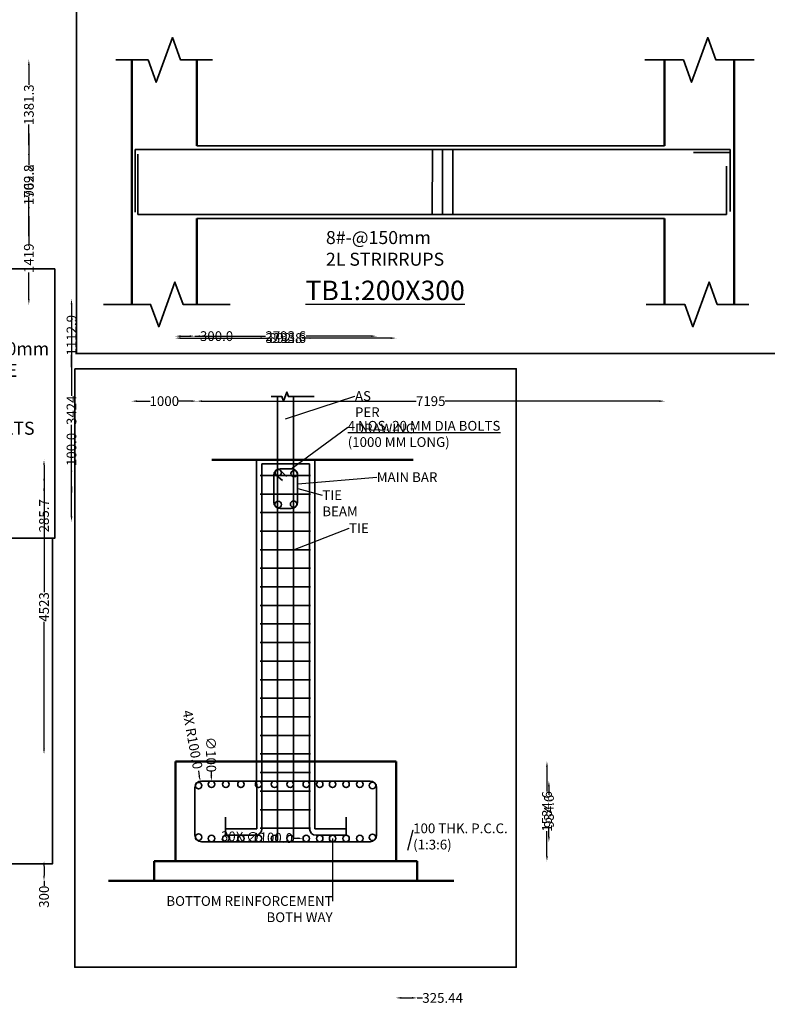
# Model space of a CAD drawing. Units: millimetres. Extents: x -19888 to 14444, y 67066 to 90098.
# Tile 3 of 7: x -9513 to 1986, y 67066 to 82214. Entities that reach past the tile are written whole.
import ezdxf
from ezdxf import colors
from ezdxf.entities.mleader import LeaderData, LeaderLine
from ezdxf.math import Vec2, Vec3

# ---------------------------------------------------------------- set-up
doc = ezdxf.new("R2010")
doc.units = ezdxf.units.MM
doc.header["$LTSCALE"] = 50
doc.header["$MEASUREMENT"] = 0
for name, color, linetype, lineweight in [('S-ANNO-DIMS', 2, 'Continuous', 18), ('S-ANNO-TEXT', 7, 'Continuous', 25), ('S-ANNO-TTLB', 7, 'Continuous', 35), ('S-BEAM', 3, 'Continuous', 35), ('S-COLS', 4, 'Continuous', 50), ('S-FNDN', 1, 'Continuous', 50), ('S-REIN', 6, 'Continuous', 35)]:
    doc.layers.add(name, color=color, linetype=linetype, lineweight=lineweight)
doc.styles.get("Standard").update_dxf_attribs({"font": 'arial.ttf'})
doc.dimstyles.get("Standard").update_dxf_attribs({"dimtxt": 150, "dimasz": 80, "dimexe": 0.18, "dimexo": 0.0625, "dimgap": 0.09, "dimtad": 0, "dimdec": 0, "dimzin": 0, "dimdsep": 46, "dimtxsty": 'Standard', "dimcen": 0.09, "dimadec": 0, "dimazin": 0, "dimtfac": 1, "dimtdec": 0, "dimtofl": 0, "dimtmove": 0, "dimatfit": 3, "dimfxl": 1, "dimfxlon": 1, "dimtolj": 1, "dimtzin": 0, "dimarcsym": 0})

# ---------------------------------------------------------------- blocks, each defined once
blk = doc.blocks.new('*D41')
at = {"layer": 'Defpoints', "color": 0, "ltscale": 50, "transparency": 16777216}
for p in [(-11742, 77917), (-8716, 77917), (-11519, 74493)]:
    blk.add_point(p, dxfattribs=at)
at = {"layer": 'S-ANNO-DIMS', "color": 0, "lineweight": -2, "ltscale": 50, "transparency": 16777216}
for p, q in [((-8717, 77917), (-8716, 77917)), ((-8716, 77837), (-8716, 76429)), ((-8716, 74573), (-8716, 75981)), ((-8717, 74493), (-8716, 74493))]:
    blk.add_line(p, q, dxfattribs=at)
at = {"layer": 'S-ANNO-DIMS', "color": 0, "ltscale": 50, "transparency": 16777216}
for points in [[(-8729, 77837), (-8703, 77837), (-8716, 77917)], [(-8729, 74573), (-8703, 74573), (-8716, 74493)]]:
    blk.add_solid(points, dxfattribs=at)
at = {"layer": 'S-ANNO-DIMS', "color": 0, "ltscale": 50, "transparency": 16777216, "insert": (-8716, 76205), "char_height": 150, "attachment_point": 5, "rotation": 90}
blk.add_mtext('\\A1;3424', dxfattribs=at)
blk = doc.blocks.new('*D42')
at = {"layer": 'Defpoints', "color": 0, "ltscale": 50, "transparency": 16777216}
for p in [(-11742, 77917), (-11219, 76804), (-8716, 76804)]:
    blk.add_point(p, dxfattribs=at)
at = {"layer": 'S-ANNO-DIMS', "color": 0, "lineweight": -2, "ltscale": 50, "transparency": 16777216}
for p, q in [((-8717, 77917), (-8716, 77917)), ((-8716, 77837), (-8716, 77665)), ((-8716, 76884), (-8716, 77056)), ((-8717, 76804), (-8716, 76804))]:
    blk.add_line(p, q, dxfattribs=at)
at = {"layer": 'S-ANNO-DIMS', "color": 0, "ltscale": 50, "transparency": 16777216}
for points in [[(-8729, 77837), (-8703, 77837), (-8716, 77917)], [(-8729, 76884), (-8703, 76884), (-8716, 76804)]]:
    blk.add_solid(points, dxfattribs=at)
at = {"layer": 'S-ANNO-DIMS', "color": 0, "ltscale": 50, "transparency": 16777216, "insert": (-8716, 77360), "char_height": 150, "attachment_point": 5, "rotation": 90}
blk.add_mtext('\\A1;1112.9', dxfattribs=at)
blk = doc.blocks.new('*D51')
at = {"layer": 'Defpoints', "color": 0, "ltscale": 50, "transparency": 16777216}
for p in [(1476, 82673), (-7789, 81597), (1476, 81597)]:
    blk.add_point(p, dxfattribs=at)
at = {"layer": 'S-ANNO-DIMS', "color": 0, "lineweight": -2, "ltscale": 50, "transparency": 16777216}
for p, q in [((-7789, 82672), (-7789, 82673)), ((-7709, 82673), (-3381, 82673)), ((1396, 82673), (-2931, 82673)), ((1476, 82672), (1476, 82673))]:
    blk.add_line(p, q, dxfattribs=at)
at = {"layer": 'S-ANNO-DIMS', "color": 0, "ltscale": 50, "transparency": 16777216}
for points in [[(-7709, 82686), (-7709, 82659), (-7789, 82673)], [(1396, 82686), (1396, 82659), (1476, 82673)]]:
    blk.add_solid(points, dxfattribs=at)
at = {"layer": 'S-ANNO-DIMS', "color": 0, "ltscale": 50, "transparency": 16777216, "insert": (-3156, 82673), "char_height": 150, "attachment_point": 5}
blk.add_mtext('\\A1;9265', dxfattribs=at)
blk = doc.blocks.new('*D52')
at = {"layer": 'Defpoints', "color": 0, "ltscale": 50, "transparency": 16777216}
for p in [(-7789, 77834), (-6789, 77834), (-6789, 76346)]:
    blk.add_point(p, dxfattribs=at)
at = {"layer": 'S-ANNO-DIMS', "color": 0, "lineweight": -2, "ltscale": 50, "transparency": 16777216}
for p, q in [((-7789, 76347), (-7789, 76346)), ((-7709, 76346), (-7505, 76346)), ((-6869, 76346), (-7072, 76346)), ((-6789, 76347), (-6789, 76346))]:
    blk.add_line(p, q, dxfattribs=at)
at = {"layer": 'S-ANNO-DIMS', "color": 0, "ltscale": 50, "transparency": 16777216}
for points in [[(-7709, 76359), (-7709, 76333), (-7789, 76346)], [(-6869, 76359), (-6869, 76333), (-6789, 76346)]]:
    blk.add_solid(points, dxfattribs=at)
at = {"layer": 'S-ANNO-DIMS', "color": 0, "ltscale": 50, "transparency": 16777216, "insert": (-7289, 76346), "char_height": 150, "attachment_point": 5}
blk.add_mtext('\\A1;1000', dxfattribs=at)
blk = doc.blocks.new('*D53')
at = {"layer": 'Defpoints', "color": 0, "ltscale": 50, "transparency": 16777216}
for p in [(-6789, 77834), (407, 77834), (407, 76346)]:
    blk.add_point(p, dxfattribs=at)
at = {"layer": 'S-ANNO-DIMS', "color": 0, "lineweight": -2, "ltscale": 50, "transparency": 16777216}
for p, q in [((-6789, 76347), (-6789, 76346)), ((-6709, 76346), (-3415, 76346)), ((327, 76346), (-2967, 76346)), ((407, 76347), (407, 76346))]:
    blk.add_line(p, q, dxfattribs=at)
at = {"layer": 'S-ANNO-DIMS', "color": 0, "ltscale": 50, "transparency": 16777216}
for points in [[(-6709, 76359), (-6709, 76333), (-6789, 76346)], [(327, 76359), (327, 76333), (407, 76346)]]:
    blk.add_solid(points, dxfattribs=at)
at = {"layer": 'S-ANNO-DIMS', "color": 0, "ltscale": 50, "transparency": 16777216, "insert": (-3191, 76346), "char_height": 150, "attachment_point": 5}
blk.add_mtext('\\A1;7195', dxfattribs=at)
blk = doc.blocks.new('*D54')
at = {"layer": 'Defpoints', "color": 0, "ltscale": 50, "transparency": 16777216}
for p in [(-7789, 81597), (-9372, 80215), (-7739, 80215)]:
    blk.add_point(p, dxfattribs=at)
at = {"layer": 'S-ANNO-DIMS', "color": 0, "lineweight": -2, "ltscale": 50, "transparency": 16777216}
for p, q in [((-9371, 81597), (-9372, 81597)), ((-9372, 81517), (-9372, 81210)), ((-9372, 80295), (-9372, 80602)), ((-9371, 80215), (-9372, 80215))]:
    blk.add_line(p, q, dxfattribs=at)
at = {"layer": 'S-ANNO-DIMS', "color": 0, "ltscale": 50, "transparency": 16777216}
for points in [[(-9385, 81517), (-9359, 81517), (-9372, 81597)], [(-9385, 80295), (-9359, 80295), (-9372, 80215)]]:
    blk.add_solid(points, dxfattribs=at)
at = {"layer": 'S-ANNO-DIMS', "color": 0, "ltscale": 50, "transparency": 16777216, "insert": (-9372, 80906), "char_height": 150, "attachment_point": 5, "rotation": 90}
blk.add_mtext('\\A1;1381.3', dxfattribs=at)
blk = doc.blocks.new('*D55')
at = {"layer": 'Defpoints', "color": 0, "ltscale": 50, "transparency": 16777216}
for p in [(-7739, 80215), (-9372, 79253), (-7739, 79253)]:
    blk.add_point(p, dxfattribs=at)
at = {"layer": 'S-ANNO-DIMS', "color": 0, "lineweight": -2, "ltscale": 50, "transparency": 16777216}
for p, q in [((-9371, 80215), (-9372, 80215)), ((-9372, 80135), (-9372, 79987)), ((-9372, 79333), (-9372, 79482)), ((-9371, 79253), (-9372, 79253))]:
    blk.add_line(p, q, dxfattribs=at)
at = {"layer": 'S-ANNO-DIMS', "color": 0, "ltscale": 50, "transparency": 16777216}
for points in [[(-9385, 80135), (-9359, 80135), (-9372, 80215)], [(-9385, 79333), (-9359, 79333), (-9372, 79253)]]:
    blk.add_solid(points, dxfattribs=at)
at = {"layer": 'S-ANNO-DIMS', "color": 0, "ltscale": 50, "transparency": 16777216, "insert": (-9372, 79734), "char_height": 150, "attachment_point": 5, "rotation": 90}
blk.add_mtext('\\A1;962.2', dxfattribs=at)
blk = doc.blocks.new('*D56')
at = {"layer": 'Defpoints', "color": 0, "ltscale": 50, "transparency": 16777216}
for p in [(-7739, 79253), (-9372, 77834), (-7789, 77834)]:
    blk.add_point(p, dxfattribs=at)
at = {"layer": 'S-ANNO-DIMS', "color": 0, "lineweight": -2, "ltscale": 50, "transparency": 16777216}
for p, q in [((-9371, 79253), (-9372, 79253)), ((-9372, 79173), (-9372, 78761)), ((-9372, 77914), (-9372, 78326)), ((-9371, 77834), (-9372, 77834))]:
    blk.add_line(p, q, dxfattribs=at)
at = {"layer": 'S-ANNO-DIMS', "color": 0, "ltscale": 50, "transparency": 16777216}
for points in [[(-9385, 79173), (-9359, 79173), (-9372, 79253)], [(-9385, 77914), (-9359, 77914), (-9372, 77834)]]:
    blk.add_solid(points, dxfattribs=at)
at = {"layer": 'S-ANNO-DIMS', "color": 0, "ltscale": 50, "transparency": 16777216, "insert": (-9372, 78544), "char_height": 150, "attachment_point": 5, "rotation": 90}
blk.add_mtext('\\A1;1419', dxfattribs=at)
blk = doc.blocks.new('*D57')
at = {"layer": 'Defpoints', "color": 0, "ltscale": 50, "transparency": 16777216}
for p in [(-3161, 82673), (-6789, 80274), (-3161, 80215)]:
    blk.add_point(p, dxfattribs=at)
at = {"layer": 'S-ANNO-DIMS', "color": 0, "lineweight": -2, "ltscale": 50, "transparency": 16777216}
for p, q in [((-6789, 82672), (-6789, 82673)), ((-6709, 82673), (-5286, 82673)), ((-3241, 82673), (-4664, 82673)), ((-3161, 82672), (-3161, 82673))]:
    blk.add_line(p, q, dxfattribs=at)
at = {"layer": 'S-ANNO-DIMS', "color": 0, "ltscale": 50, "transparency": 16777216}
for points in [[(-6709, 82686), (-6709, 82659), (-6789, 82673)], [(-3241, 82686), (-3241, 82659), (-3161, 82673)]]:
    blk.add_solid(points, dxfattribs=at)
at = {"layer": 'S-ANNO-DIMS', "color": 0, "ltscale": 50, "transparency": 16777216, "insert": (-4975, 82673), "char_height": 150, "attachment_point": 5}
blk.add_mtext('\\A1;3627.4', dxfattribs=at)
blk = doc.blocks.new('*D59')
at = {"layer": 'Defpoints', "color": 0, "ltscale": 50, "transparency": 16777216}
for p in [(2744, 80527), (-9372, 78817), (2744, 78817)]:
    blk.add_point(p, dxfattribs=at)
at = {"layer": 'S-ANNO-DIMS', "color": 0, "lineweight": -2, "ltscale": 50, "transparency": 16777216}
for p, q in [((-9371, 80527), (-9372, 80527)), ((-9372, 80447), (-9372, 79976)), ((-9372, 78897), (-9372, 79367)), ((-9371, 78817), (-9372, 78817))]:
    blk.add_line(p, q, dxfattribs=at)
at = {"layer": 'S-ANNO-DIMS', "color": 0, "ltscale": 50, "transparency": 16777216}
for points in [[(-9385, 80447), (-9359, 80447), (-9372, 80527)], [(-9385, 78897), (-9359, 78897), (-9372, 78817)]]:
    blk.add_solid(points, dxfattribs=at)
at = {"layer": 'S-ANNO-DIMS', "color": 0, "ltscale": 50, "transparency": 16777216, "insert": (-9372, 79672), "char_height": 150, "attachment_point": 5, "rotation": 90}
blk.add_mtext('\\A1;1709.8', dxfattribs=at)
blk = doc.blocks.new('*D61')
at = {"layer": 'Defpoints', "color": 0, "ltscale": 50, "transparency": 16777216}
for p in [(-3725, 77316), (-7118, 70801), (-3725, 70801)]:
    blk.add_point(p, dxfattribs=at)
at = {"layer": 'S-ANNO-DIMS', "color": 0, "lineweight": -2, "ltscale": 50, "transparency": 16777216}
for p, q in [((-7118, 77315), (-7118, 77316)), ((-7038, 77316), (-5733, 77316)), ((-3805, 77316), (-5110, 77316)), ((-3725, 77315), (-3725, 77316))]:
    blk.add_line(p, q, dxfattribs=at)
at = {"layer": 'S-ANNO-DIMS', "color": 0, "ltscale": 50, "transparency": 16777216}
for points in [[(-7038, 77329), (-7038, 77302), (-7118, 77316)], [(-3805, 77329), (-3805, 77302), (-3725, 77316)]]:
    blk.add_solid(points, dxfattribs=at)
at = {"layer": 'S-ANNO-DIMS', "color": 0, "ltscale": 50, "transparency": 16777216, "insert": (-5421, 77316), "char_height": 150, "attachment_point": 5}
blk.add_mtext('\\A1;3393.6', dxfattribs=at)
blk = doc.blocks.new('*D62')
at = {"layer": 'Defpoints', "color": 0, "ltscale": 50, "transparency": 16777216}
for p in [(-3725, 69267), (-3399, 69267), (-3399, 67164)]:
    blk.add_point(p, dxfattribs=at)
at = {"layer": 'S-ANNO-DIMS', "color": 0, "lineweight": -2, "ltscale": 50, "transparency": 16777216}
for p, q in [((-3725, 67165), (-3725, 67164)), ((-3645, 67164), (-3479, 67164)), ((-3399, 67165), (-3399, 67164)), ((-3399, 67164), (-3319, 67164))]:
    blk.add_line(p, q, dxfattribs=at)
at = {"layer": 'S-ANNO-DIMS', "color": 0, "ltscale": 50, "transparency": 16777216}
for points in [[(-3645, 67178), (-3645, 67151), (-3725, 67164)], [(-3479, 67178), (-3479, 67151), (-3399, 67164)]]:
    blk.add_solid(points, dxfattribs=at)
at = {"layer": 'S-ANNO-DIMS', "color": 0, "ltscale": 50, "transparency": 16777216, "insert": (-3008, 67164), "char_height": 150, "attachment_point": 5}
blk.add_mtext('\\A1;325.44', dxfattribs=at)
blk = doc.blocks.new('*D63')
at = {"layer": 'Defpoints', "color": 0, "ltscale": 50, "transparency": 16777216}
for p in [(-4975, 77316), (-5868, 69767), (-4975, 69767)]:
    blk.add_point(p, dxfattribs=at)
at = {"layer": 'S-ANNO-DIMS', "color": 0, "lineweight": -2, "ltscale": 50, "transparency": 16777216}
for p, q in [((-5868, 77315), (-5868, 77316)), ((-5788, 77316), (-5675, 77316)), ((-5055, 77316), (-5168, 77316)), ((-4975, 77315), (-4975, 77316))]:
    blk.add_line(p, q, dxfattribs=at)
at = {"layer": 'S-ANNO-DIMS', "color": 0, "ltscale": 50, "transparency": 16777216}
for points in [[(-5788, 77329), (-5788, 77302), (-5868, 77316)], [(-5055, 77329), (-5055, 77302), (-4975, 77316)]]:
    blk.add_solid(points, dxfattribs=at)
at = {"layer": 'S-ANNO-DIMS', "color": 0, "ltscale": 50, "transparency": 16777216, "insert": (-5421, 77316), "char_height": 150, "attachment_point": 5}
blk.add_mtext('\\A1;892.8', dxfattribs=at)
blk = doc.blocks.new('*D64')
at = {"layer": 'Defpoints', "color": 0, "ltscale": 50, "transparency": 16777216}
for p in [(-3725, 70801), (-3725, 69267), (-1403, 69267)]:
    blk.add_point(p, dxfattribs=at)
at = {"layer": 'S-ANNO-DIMS', "color": 0, "lineweight": -2, "ltscale": 50, "transparency": 16777216}
for p, q in [((-1404, 70801), (-1403, 70801)), ((-1403, 70721), (-1403, 70338)), ((-1403, 69347), (-1403, 69730)), ((-1404, 69267), (-1403, 69267))]:
    blk.add_line(p, q, dxfattribs=at)
at = {"layer": 'S-ANNO-DIMS', "color": 0, "ltscale": 50, "transparency": 16777216}
for points in [[(-1417, 70721), (-1390, 70721), (-1403, 70801)], [(-1417, 69347), (-1390, 69347), (-1403, 69267)]]:
    blk.add_solid(points, dxfattribs=at)
at = {"layer": 'S-ANNO-DIMS', "color": 0, "ltscale": 50, "transparency": 16777216, "insert": (-1403, 70034), "char_height": 150, "attachment_point": 5, "rotation": 90}
blk.add_mtext('\\A1;1534.6', dxfattribs=at)
blk = doc.blocks.new('*D65')
at = {"layer": 'Defpoints', "color": 0, "ltscale": 50, "transparency": 16777216}
for p in [(-7444, 69267), (-9139, 68967), (-7444, 68967)]:
    blk.add_point(p, dxfattribs=at)
at = {"layer": 'S-ANNO-DIMS', "color": 0, "lineweight": -2, "ltscale": 50, "transparency": 16777216}
for p, q in [((-9138, 69267), (-9139, 69267)), ((-9139, 69187), (-9139, 69047)), ((-9138, 68967), (-9139, 68967)), ((-9139, 68967), (-9139, 68887))]:
    blk.add_line(p, q, dxfattribs=at)
at = {"layer": 'S-ANNO-DIMS', "color": 0, "ltscale": 50, "transparency": 16777216}
for points in [[(-9152, 69187), (-9126, 69187), (-9139, 69267)], [(-9152, 69047), (-9126, 69047), (-9139, 68967)]]:
    blk.add_solid(points, dxfattribs=at)
at = {"layer": 'S-ANNO-DIMS', "color": 0, "ltscale": 50, "transparency": 16777216, "insert": (-9139, 68721), "char_height": 150, "attachment_point": 5, "rotation": 90}
blk.add_mtext('\\A1;300', dxfattribs=at)
blk = doc.blocks.new('*D66')
at = {"layer": 'Defpoints', "color": 0, "ltscale": 50, "transparency": 16777216}
for p in [(-5868, 75441), (-9139, 70917), (-5814, 70917)]:
    blk.add_point(p, dxfattribs=at)
at = {"layer": 'S-ANNO-DIMS', "color": 0, "lineweight": -2, "ltscale": 50, "transparency": 16777216}
for p, q in [((-9138, 75441), (-9139, 75441)), ((-9139, 75361), (-9139, 73406)), ((-9139, 70997), (-9139, 72952)), ((-9138, 70917), (-9139, 70917))]:
    blk.add_line(p, q, dxfattribs=at)
at = {"layer": 'S-ANNO-DIMS', "color": 0, "ltscale": 50, "transparency": 16777216}
for points in [[(-9152, 75361), (-9126, 75361), (-9139, 75441)], [(-9152, 70997), (-9126, 70997), (-9139, 70917)]]:
    blk.add_solid(points, dxfattribs=at)
at = {"layer": 'S-ANNO-DIMS', "color": 0, "ltscale": 50, "transparency": 16777216, "insert": (-9139, 73179), "char_height": 150, "attachment_point": 5, "rotation": 90}
blk.add_mtext('\\A1;4523', dxfattribs=at)
blk = doc.blocks.new('*D67')
at = {"layer": 'Defpoints', "color": 0, "ltscale": 50, "transparency": 16777216}
for p in [(-5814, 75202), (-9139, 74917), (-5814, 74917)]:
    blk.add_point(p, dxfattribs=at)
at = {"layer": 'S-ANNO-DIMS', "color": 0, "lineweight": -2, "ltscale": 50, "transparency": 16777216}
for p, q in [((-9138, 75202), (-9139, 75202)), ((-9139, 75122), (-9139, 74997)), ((-9138, 74917), (-9139, 74917)), ((-9139, 74917), (-9139, 74837))]:
    blk.add_line(p, q, dxfattribs=at)
at = {"layer": 'S-ANNO-DIMS', "color": 0, "ltscale": 50, "transparency": 16777216}
for points in [[(-9152, 75122), (-9126, 75122), (-9139, 75202)], [(-9152, 74997), (-9126, 74997), (-9139, 74917)]]:
    blk.add_solid(points, dxfattribs=at)
at = {"layer": 'S-ANNO-DIMS', "color": 0, "ltscale": 50, "transparency": 16777216, "insert": (-9139, 74582), "char_height": 150, "attachment_point": 5, "rotation": 90}
blk.add_mtext('\\A1;285.7', dxfattribs=at)
blk = doc.blocks.new('*D71')
at = {"layer": 'Defpoints', "color": 0, "ltscale": 50, "transparency": 16777216}
for p in [(-6564, 70501), (-6563, 70401)]:
    blk.add_point(p, dxfattribs=at)
at = {"layer": 'S-ANNO-DIMS', "color": 0, "lineweight": -2, "ltscale": 50, "transparency": 16777216}
for p, q in [((-6567, 70661), (-6566, 70581)), ((-6564, 70451), (-6563, 70451)), ((-6564, 70451), (-6564, 70451))]:
    blk.add_line(p, q, dxfattribs=at)
at = {"layer": 'S-ANNO-DIMS', "color": 0, "ltscale": 50, "transparency": 16777216}
blk.add_solid([(-6552, 70581), (-6579, 70581), (-6564, 70501)], dxfattribs=at)
at = {"layer": 'S-ANNO-DIMS', "color": 0, "ltscale": 50, "transparency": 16777216, "insert": (-6570, 70908), "char_height": 150, "attachment_point": 5, "rotation": 270.8674}
blk.add_mtext('\\A1;∅100', dxfattribs=at)
blk = doc.blocks.new('*D94')
at = {"layer": 'Defpoints', "color": 0, "ltscale": 50, "transparency": 16777216}
for p in [(-11369, 75198), (-8716, 75198), (-11369, 75098)]:
    blk.add_point(p, dxfattribs=at)
at = {"layer": 'S-ANNO-DIMS', "color": 0, "lineweight": -2, "ltscale": 50, "transparency": 16777216}
for p, q in [((-8716, 75278), (-8716, 75358)), ((-8717, 75198), (-8716, 75198)), ((-8717, 75098), (-8716, 75098)), ((-8716, 75018), (-8716, 74938))]:
    blk.add_line(p, q, dxfattribs=at)
at = {"layer": 'S-ANNO-DIMS', "color": 0, "ltscale": 50, "transparency": 16777216}
for points in [[(-8729, 75278), (-8703, 75278), (-8716, 75198)], [(-8729, 75018), (-8703, 75018), (-8716, 75098)]]:
    blk.add_solid(points, dxfattribs=at)
at = {"layer": 'S-ANNO-DIMS', "color": 0, "ltscale": 50, "transparency": 16777216, "insert": (-8716, 75603), "char_height": 150, "attachment_point": 5, "rotation": 90}
blk.add_mtext('\\A1;100.0', dxfattribs=at)
blk = doc.blocks.new('*D97')
at = {"layer": 'Defpoints', "color": 0, "ltscale": 50, "transparency": 16777216}
for p in [(-4025, 77346), (-6818, 70401), (-4025, 70401)]:
    blk.add_point(p, dxfattribs=at)
at = {"layer": 'S-ANNO-DIMS', "color": 0, "lineweight": -2, "ltscale": 50, "transparency": 16777216}
for p, q in [((-6818, 77345), (-6818, 77346)), ((-6738, 77346), (-5734, 77346)), ((-4105, 77346), (-5109, 77346)), ((-4025, 77345), (-4025, 77346))]:
    blk.add_line(p, q, dxfattribs=at)
at = {"layer": 'S-ANNO-DIMS', "color": 0, "ltscale": 50, "transparency": 16777216}
for points in [[(-6738, 77359), (-6738, 77332), (-6818, 77346)], [(-4105, 77359), (-4105, 77332), (-4025, 77346)]]:
    blk.add_solid(points, dxfattribs=at)
at = {"layer": 'S-ANNO-DIMS', "color": 0, "ltscale": 50, "transparency": 16777216, "insert": (-5421, 77346), "char_height": 150, "attachment_point": 5}
blk.add_mtext('\\A1;2793.6', dxfattribs=at)
blk = doc.blocks.new('*D98')
at = {"layer": 'Defpoints', "color": 0, "ltscale": 50, "transparency": 16777216}
for p in [(-4125, 70501), (-4125, 69567), (-1373, 69567)]:
    blk.add_point(p, dxfattribs=at)
at = {"layer": 'S-ANNO-DIMS', "color": 0, "lineweight": -2, "ltscale": 50, "transparency": 16777216}
for p, q in [((-1374, 70501), (-1373, 70501)), ((-1373, 70421), (-1373, 70287)), ((-1373, 69647), (-1373, 69781)), ((-1374, 69567), (-1373, 69567))]:
    blk.add_line(p, q, dxfattribs=at)
at = {"layer": 'S-ANNO-DIMS', "color": 0, "ltscale": 50, "transparency": 16777216}
for points in [[(-1387, 70421), (-1360, 70421), (-1373, 70501)], [(-1387, 69647), (-1360, 69647), (-1373, 69567)]]:
    blk.add_solid(points, dxfattribs=at)
at = {"layer": 'S-ANNO-DIMS', "color": 0, "ltscale": 50, "transparency": 16777216, "insert": (-1373, 70034), "char_height": 150, "attachment_point": 5, "rotation": 90}
blk.add_mtext('\\A1;934.6', dxfattribs=at)
blk = doc.blocks.new('*D99')
at = {"layer": 'Defpoints', "color": 0, "ltscale": 50, "transparency": 16777216}
for p in [(-6818, 77346), (-7118, 70801), (-6818, 70401)]:
    blk.add_point(p, dxfattribs=at)
at = {"layer": 'S-ANNO-DIMS', "color": 0, "lineweight": -2, "ltscale": 50, "transparency": 16777216}
for p, q in [((-7118, 77345), (-7118, 77346)), ((-7038, 77346), (-6898, 77346)), ((-6818, 77345), (-6818, 77346)), ((-6818, 77346), (-6738, 77346))]:
    blk.add_line(p, q, dxfattribs=at)
at = {"layer": 'S-ANNO-DIMS', "color": 0, "ltscale": 50, "transparency": 16777216}
for points in [[(-7038, 77359), (-7038, 77332), (-7118, 77346)], [(-6898, 77359), (-6898, 77332), (-6818, 77346)]]:
    blk.add_solid(points, dxfattribs=at)
at = {"layer": 'S-ANNO-DIMS', "color": 0, "ltscale": 50, "transparency": 16777216, "insert": (-6485, 77346), "char_height": 150, "attachment_point": 5}
blk.add_mtext('\\A1;300.0', dxfattribs=at)
blk = doc.blocks.new('*D105')
at = {"layer": 'Defpoints', "color": 0, "ltscale": 50, "transparency": 16777216}
for p in [(-5155, 69618), (-5055, 69615)]:
    blk.add_point(p, dxfattribs=at)
at = {"layer": 'S-ANNO-DIMS', "color": 0, "lineweight": -2, "ltscale": 50, "transparency": 16777216}
for p, q in [((-5315, 69623), (-5235, 69620)), ((-5105, 69617), (-5105, 69617)), ((-5105, 69617), (-5105, 69617))]:
    blk.add_line(p, q, dxfattribs=at)
at = {"layer": 'S-ANNO-DIMS', "color": 0, "ltscale": 50, "transparency": 16777216}
blk.add_solid([(-5235, 69634), (-5235, 69607), (-5155, 69618)], dxfattribs=at)
at = {"layer": 'S-ANNO-DIMS', "color": 0, "ltscale": 50, "transparency": 16777216, "insert": (-5865, 69638), "char_height": 150, "attachment_point": 5, "rotation": 358.3831}
blk.add_mtext('\\A1;30X ∅100.0', dxfattribs=at)
blk = doc.blocks.new('*D106')
at = {"layer": 'Defpoints', "color": 0, "ltscale": 50, "transparency": 16777216}
for p in [(-6736, 70500), (-6718, 70401)]:
    blk.add_point(p, dxfattribs=at)
at = {"layer": 'S-ANNO-DIMS', "color": 0, "lineweight": -2, "ltscale": 50, "transparency": 16777216}
for p, q in [((-6765, 70657), (-6751, 70578)), ((-6718, 70401), (-6718, 70401)), ((-6718, 70401), (-6718, 70401))]:
    blk.add_line(p, q, dxfattribs=at)
at = {"layer": 'S-ANNO-DIMS', "color": 0, "ltscale": 50, "transparency": 16777216}
blk.add_solid([(-6738, 70581), (-6764, 70576), (-6736, 70500)], dxfattribs=at)
at = {"layer": 'S-ANNO-DIMS', "color": 0, "ltscale": 50, "transparency": 16777216, "insert": (-6854, 71138), "char_height": 150, "attachment_point": 5, "rotation": 280.4298}
blk.add_mtext('\\A1;4X R100.0', dxfattribs=at)

msp = doc.modelspace()

# ---------------------------------------------------------------- linework, layer by layer
at = {"layer": 'S-ANNO-TTLB', "ltscale": 50}
for points in [[(-8639.597, 82452.304), (5654.103, 82452.304), (5654.103, 77078.62), (-8639.597, 77078.62)], [(-14066.3, 78381.341), (-8972.922, 78381.341), (-8972.922, 74235.431), (-14066.3, 74235.431)], [(-8666.614, 76843.183), (-1875.715, 76843.183), (-1875.715, 67636.782), (-8666.614, 67636.782)], [(-13491.006, 74235.431), (-9009.653, 74235.431), (-9009.653, 69226.696), (-13491.006, 69226.696)]]:
    msp.add_lwpolyline(points, close=True, dxfattribs=at)
at = {"layer": 'S-BEAM', "ltscale": 50}
for p, q in [((406.717, 80274.282), (-6788.546, 80274.282)), ((406.717, 79156.947), (-6788.546, 79156.947))]:
    msp.add_line(p, q, dxfattribs=at)
for points in [[(-8032.958, 81596.699), (-7539.014, 81596.699), (-7414.014, 81253.264), (-7164.014, 81940.134), (-7039.014, 81596.699), (-6545.069, 81596.699)], [(104.104, 81596.699), (695.202, 81596.699), (820.202, 81253.264), (1070.202, 81940.134), (1195.202, 81596.699), (1786.299, 81596.699)], [(-6277.83, 77834.019), (-6999.957, 77834.019), (-7124.957, 78177.454), (-7374.957, 77490.585), (-7499.957, 77834.019), (-8222.084, 77834.019)], [(122.278, 77834.019), (716.565, 77834.019), (841.565, 77490.585), (1091.565, 78177.454), (1216.565, 77834.019), (1700.586, 77834.019)]]:
    msp.add_lwpolyline(points, dxfattribs=at)
at = {"layer": 'S-COLS', "ltscale": 50}
for p, q in [((-7788.546, 81596.699), (-7788.546, 77834.019)), ((-6788.546, 81596.699), (-6788.546, 80274.282)), ((406.717, 81596.699), (406.717, 80274.282)), ((1476.348, 81596.699), (1476.348, 77834.019)), ((-6788.546, 79156.947), (-6788.546, 77834.019)), ((406.717, 79156.947), (406.717, 77834.019))]:
    msp.add_line(p, q, dxfattribs=at)
at = {"layer": 'S-FNDN', "ltscale": 50}
for p, q in [((-6556.198, 75440.577), (-3462.409, 75440.577)), ((-7118.183, 69855.095), (-7118.183, 70801.206)), ((-7118.183, 70801.206), (-3724.562, 70801.206)), ((-3724.562, 70801.206), (-3724.562, 69266.644)), ((-7118.183, 69266.644), (-7118.183, 69855.095)), ((-3399.12, 69266.644), (-7443.625, 69266.644)), ((-7443.625, 69266.644), (-7443.625, 68966.644)), ((-3399.12, 68966.644), (-3399.12, 69266.644)), ((-8149.449, 68966.644), (-2837.132, 68966.644))]:
    msp.add_line(p, q, dxfattribs=at)
at = {"layer": 'S-REIN', "ltscale": 50}
for p, q in [((-7738.799, 80215.359), (1416.444, 80215.359)), ((-7738.799, 80215.359), (-7738.799, 79253.116)), ((-7693.752, 79215.359), (-7693.752, 80146.51)), ((-3161.177, 80215.359), (-3166.922, 79215.359)), ((-3007.78, 80215.359), (-3007.78, 79215.359)), ((-2849.469, 80215.359), (-2849.469, 79215.359)), ((1416.444, 80171.229), (849.61, 80171.229)), ((1416.444, 80215.359), (1416.444, 79264.226)), ((1359.908, 79215.359), (1359.908, 79961.611)), ((-7693.752, 79215.359), (1359.908, 79215.359)), ((-5545.216, 75710.292), (-5545.216, 76415.921)), ((-5302.113, 75771.092), (-5302.113, 76415.921)), ((-5302.113, 69616.644), (-5302.113, 75771.092)), ((-5545.216, 69616.644), (-5545.216, 75710.292)), ((-5868.32, 70451.206), (-5868.32, 75440.577)), ((-4974.957, 70451.206), (-4974.957, 75440.577)), ((-5788.32, 70451.206), (-5788.32, 75378.848)), ((-5054.957, 75378.848), (-5788.32, 75378.848)), ((-5054.957, 70451.206), (-5054.957, 75378.848)), ((-5038.983, 75202.484), (-5813.701, 75202.484)), ((-5567.613, 75207.322), (-5468.681, 75125.25)), ((-5500.133, 75280.958), (-5406.737, 75186.493)), ((-5038.983, 74916.811), (-5813.701, 74916.811)), ((-5038.983, 74631.137), (-5813.701, 74631.137)), ((-5038.983, 74345.463), (-5813.701, 74345.463)), ((-5038.983, 74059.789), (-5813.701, 74059.789)), ((-5038.983, 73774.115), (-5813.701, 73774.115)), ((-5038.983, 73488.441), (-5813.701, 73488.441)), ((-5038.983, 73202.767), (-5813.701, 73202.767)), ((-5038.983, 72917.093), (-5813.701, 72917.093)), ((-5038.983, 72631.419), (-5813.701, 72631.419)), ((-5038.983, 72345.745), (-5813.701, 72345.745)), ((-5038.983, 72060.071), (-5813.701, 72060.071)), ((-5038.983, 71774.397), (-5813.701, 71774.397)), ((-5038.983, 71488.723), (-5813.701, 71488.723)), ((-5038.983, 71203.049), (-5813.701, 71203.049)), ((-5038.983, 70917.375), (-5813.701, 70917.375)), ((-5038.983, 70631.701), (-5813.701, 70631.701)), ((-6718.183, 70501.206), (-4124.562, 70501.206)), ((-5867.788, 70451.206), (-5867.788, 69766.644)), ((-5787.788, 70451.206), (-5787.788, 69766.644)), ((-5054.957, 70451.206), (-5054.957, 69766.644)), ((-4974.957, 70451.206), (-4974.957, 69766.644)), ((-6818.183, 69855.095), (-6818.183, 70401.206)), ((-5038.983, 70346.027), (-5813.701, 70346.027)), ((-4024.562, 70401.206), (-4024.562, 69666.644)), ((-5038.983, 70060.353), (-5813.701, 70060.353)), ((-6818.183, 69666.644), (-6818.183, 69855.095)), ((-6349.599, 69666.644), (-6349.599, 69946.149)), ((-4493.146, 69666.644), (-4493.146, 69946.149)), ((-5867.788, 69766.644), (-6349.599, 69766.644)), ((-5038.983, 69774.68), (-5813.701, 69774.68)), ((-4974.957, 69766.644), (-4493.146, 69766.644)), ((-4124.562, 69566.644), (-6718.183, 69566.644)), ((-5887.788, 69666.644), (-6349.599, 69666.644)), ((-4954.957, 69666.644), (-4493.146, 69666.644))]:
    msp.add_line(p, q, dxfattribs=at)
msp.add_lwpolyline([(-5646.555, 76415.921), (-5478.851, 76415.921), (-5453.851, 76347.234), (-5403.851, 76484.608), (-5378.851, 76415.921), (-4983.263, 76415.921)], dxfattribs=at)
msp.add_lwpolyline([(-5504.997, 75305.069), (-5337.584, 75305.069, -0.414213562), (-5237.584, 75205.069), (-5237.584, 74793.487, -0.414213562), (-5337.584, 74693.487), (-5504.997, 74693.487, -0.414213562), (-5604.997, 74793.487), (-5604.997, 75205.069, -0.414213562)], format="xyb", close=True, dxfattribs=at)
for centre in [(-5535.689, 75245.804), (-5292.113, 75230.249), (-5538.727, 74756.381), (-5299.535, 74761.044), (-6761.025, 70430.404), (-6563.579, 70451.206), (-6341.515, 70451.206), (-6109.786, 70451.206), (-5838.32, 70451.206), (-5595.216, 70451.206), (-5352.113, 70451.206), (-5104.957, 70451.206), (-4898.319, 70451.206), (-4699.784, 70451.206), (-4493.146, 70451.206), (-4282.456, 70451.206), (-4085.714, 70433.384), (-6761.025, 69637.446), (-4085.714, 69634.466), (-6563.579, 69616.644), (-6341.515, 69616.644), (-6109.786, 69616.644), (-5838.32, 69616.644), (-5595.216, 69616.644), (-5352.113, 69616.644), (-5104.957, 69616.644), (-4898.319, 69616.644), (-4699.784, 69616.644), (-4493.146, 69616.644), (-4282.456, 69616.644)]:
    msp.add_circle(centre, 50, dxfattribs=at)
for centre, start, end in [((-6718.183, 70401.206), 90, 180), ((-4124.562, 70401.206), 0, 90), ((-5887.788, 69766.644), 270, 0), ((-4954.957, 69766.644), 180, 270), ((-6718.183, 69666.644), 180, 270), ((-4124.562, 69666.644), 270, 0)]:
    msp.add_arc(centre, 100, start, end, dxfattribs=at)

# ---------------------------------------------------------------- texts
at = {"layer": 'S-ANNO-TEXT', "ltscale": 50, "attachment_point": 1}
for s, width, heights, insert, char_height in [('8#-@150mm\\P2L STRIRRUPS', 2263.41642, [0], (-4803.069, 78962.613), 200), ('{\\LTB1:200X300}', 3602.83103, [365.321], (-5118.788, 78199.34), 300), ('300X300X20mm\\PBASE PLATE', 2233.4119, [0], (-11088.137, 77252.773), 200), ('{\\L4 NO.-20 BO}LTS\\P1000 mm LG', 2263.41642, [0], (-11286.71, 76028.76), 200)]:
    msp.add_mtext_dynamic_manual_height_columns(s, width=width, gutter_width=1, heights=heights, dxfattribs=dict(at, insert=insert, char_height=char_height))

# ---------------------------------------------------------------- dimensions: what is measured, and where the dimension line sits
at = {"layer": 'S-ANNO-DIMS', "ltscale": 50}
for base, p1, p2, override, picture, middle in [((1476.348, 82672.634), (-7788.546, 81596.699), (1476.348, 81596.699), {"dimdec": 0, "dimlfac": 1, "dimrnd": 0, "dimzin": 0, "dimdsep": 46, "dimlunit": 2}, '*D51', (-3156.099, 82672.634)), ((-3161.177, 82672.634), (-6788.546, 80274.282), (-3161.177, 80215.359), {"dimdec": 1, "dimlfac": 1, "dimrnd": 0, "dimzin": 0, "dimdsep": 46, "dimlunit": 2}, '*D57', (-4974.862, 82672.634)), ((-6788.546, 76346.12), (-7788.546, 77834.019), (-6788.546, 77834.019), {"dimdec": 0, "dimlfac": 1, "dimrnd": 0, "dimzin": 0, "dimdsep": 46, "dimlunit": 2}, '*D52', (-7288.546, 76346.12)), ((406.717, 76346.12), (-6788.546, 77834.019), (406.717, 77834.019), {"dimdec": 0, "dimlfac": 1, "dimrnd": 0, "dimzin": 0, "dimdsep": 46, "dimlunit": 2}, '*D53', (-3190.914, 76346.12)), ((-6818.183, 77345.683), (-7118.183, 70801.206), (-6818.183, 70401.206), {"dimdec": 1, "dimlfac": 1, "dimrnd": 0, "dimzin": 0, "dimdsep": 46, "dimlunit": 2}, '*D99', (-6485.313, 77345.683)), ((-3724.562, 77315.683), (-7118.183, 70801.206), (-3724.562, 70801.206), {"dimdec": 1, "dimlfac": 1, "dimrnd": 0, "dimzin": 0, "dimdsep": 46, "dimlunit": 2}, '*D61', (-5421.372, 77315.683)), ((-4024.562, 77345.683), (-6818.183, 70401.206), (-4024.562, 70401.206), {"dimdec": 1, "dimlfac": 1, "dimrnd": 0, "dimzin": 0, "dimdsep": 46, "dimlunit": 2}, '*D97', (-5421.372, 77345.683)), ((-4974.957, 77315.683), (-5867.788, 69766.644), (-4974.957, 69766.644), {"dimdec": 1, "dimlfac": 1, "dimrnd": 0, "dimzin": 0, "dimdsep": 46, "dimlunit": 2}, '*D63', (-5421.372, 77315.683)), ((-3399.12, 67164.282), (-3724.562, 69266.644), (-3399.12, 69266.644), {"dimdec": 2, "dimlfac": 1, "dimrnd": 0, "dimzin": 0, "dimdsep": 46, "dimlunit": 2}, '*D62', (-3008.03, 67164.282))]:
    dim = msp.add_linear_dim(base=base, p1=p1, p2=p2, dimstyle='Standard', override=override, dxfattribs=at)
    dim.commit()
    dim.dimension.update_dxf_attribs({"geometry": picture, "text_midpoint": middle})
for base, p1, p2, override, picture, middle in [((-9372.097, 80215.359), (-7788.546, 81596.699), (-7738.799, 80215.359), {"dimdec": 1, "dimlfac": 1, "dimrnd": 0, "dimzin": 0, "dimdsep": 46, "dimlunit": 2}, '*D54', (-9372.097, 80906.029)), ((-9372.097, 78816.838), (2743.808, 80526.651), (2743.808, 78816.838), {"dimdec": 1, "dimlfac": 1, "dimrnd": 0, "dimzin": 0, "dimdsep": 46, "dimlunit": 2}, '*D59', (-9372.097, 79671.745)), ((-9372.097, 79253.116), (-7738.799, 80215.359), (-7738.799, 79253.116), {"dimdec": 1, "dimlfac": 1, "dimrnd": 0, "dimzin": 0, "dimdsep": 46, "dimlunit": 2}, '*D55', (-9372.097, 79734.238)), ((-9372.097, 77834.019), (-7738.799, 79253.116), (-7788.546, 77834.019), {"dimdec": 0, "dimlfac": 1, "dimrnd": 0, "dimzin": 0, "dimdsep": 46, "dimlunit": 2}, '*D56', (-9372.097, 78543.568)), ((-8715.922, 77916.725), (-11518.513, 74493.06), (-11742.33, 77916.725), {"dimdec": 0, "dimlfac": 1, "dimrnd": 0, "dimzin": 0, "dimdsep": 46, "dimlunit": 2}, '*D41', (-8715.922, 76204.893)), ((-8715.922, 76803.857), (-11742.33, 77916.725), (-11218.513, 76803.857), {"dimdec": 1, "dimlfac": 1, "dimrnd": 0, "dimzin": 0, "dimdsep": 46, "dimlunit": 2}, '*D42', (-8715.922, 77360.291)), ((-8715.922, 75197.57), (-11368.513, 75097.57), (-11368.513, 75197.57), {"dimdec": 1, "dimlfac": 1, "dimrnd": 0, "dimzin": 0, "dimdsep": 46, "dimlunit": 2}, '*D94', (-8715.922, 75603.431)), ((-9139.114, 70917.375), (-5868.32, 75440.577), (-5813.701, 70917.375), {"dimdec": 0, "dimlfac": 1, "dimrnd": 0, "dimzin": 0, "dimdsep": 46, "dimlunit": 2}, '*D66', (-9139.114, 73178.976)), ((-9139.114, 74916.811), (-5813.701, 75202.484), (-5813.701, 74916.811), {"dimdec": 1, "dimlfac": 1, "dimrnd": 0, "dimzin": 0, "dimdsep": 46, "dimlunit": 2}, '*D67', (-9139.114, 74582.355)), ((-1403.215, 69266.644), (-3724.562, 70801.206), (-3724.562, 69266.644), {"dimdec": 1, "dimlfac": 1, "dimrnd": 0, "dimzin": 0, "dimdsep": 46, "dimlunit": 2}, '*D64', (-1403.215, 70033.925)), ((-1373.215, 69566.644), (-4124.562, 70501.206), (-4124.562, 69566.644), {"dimdec": 1, "dimlfac": 1, "dimrnd": 0, "dimzin": 0, "dimdsep": 46, "dimlunit": 2}, '*D98', (-1373.215, 70033.925)), ((-9139.114, 68966.644), (-7443.625, 69266.644), (-7443.625, 68966.644), {"dimdec": 0, "dimlfac": 1, "dimrnd": 0, "dimzin": 0, "dimdsep": 46, "dimlunit": 2}, '*D65', (-9139.114, 68721.155))]:
    dim = msp.add_linear_dim(base=base, p1=p1, p2=p2, angle=90, dimstyle='Standard', override=override, dxfattribs=at)
    dim.commit()
    dim.dimension.update_dxf_attribs({"geometry": picture, "text_midpoint": middle})
dim = msp.add_radius_dim(center=(-6718.183, 70401.206), mpoint=(-6736.286, 70499.554), text='4X <>', dimstyle='Standard', override={"dimdec": 1, "dimlfac": 1, "dimrnd": 0, "dimzin": 0, "dimdsep": 46, "dimlunit": 2}, dxfattribs=at)
dim.commit()
dim.dimension.update_dxf_attribs({"geometry": '*D106', "text_midpoint": (-6853.752, 71137.702)})
dim = msp.add_diameter_dim_2p(p1=(-6562.822, 70401.212), p2=(-6564.336, 70501.201), dimstyle='Standard', override={"dimdec": 0, "dimlfac": 1, "dimrnd": 0, "dimzin": 0, "dimdsep": 46, "dimlunit": 2}, dxfattribs=at)
dim.commit()
dim.dimension.update_dxf_attribs({"geometry": '*D71', "text_midpoint": (-6570.499, 70908.294)})
dim = msp.add_diameter_dim_2p(p1=(-5054.977, 69615.233), p2=(-5154.937, 69618.055), text='30X <>', dimstyle='Standard', override={"dimdec": 1, "dimlfac": 1, "dimrnd": 0, "dimzin": 0, "dimdsep": 46, "dimlunit": 2}, dxfattribs=at)
dim.commit()
dim.dimension.update_dxf_attribs({"geometry": '*D105', "text_midpoint": (-5864.557, 69638.085), "dimtype": 163})

# ---------------------------------------------------------------- leaders
at = {"layer": 'S-ANNO-TEXT', "ltscale": 50}
ml = msp.add_multileader_mtext('Standard', dxfattribs=at)
ml.set_content('\\pxt11;AS PER DRAWING', color=256)
ml.set_leader_properties()
ml.build(insert=Vec2(0, 0))
ml.multileader.update_dxf_attribs({"dogleg_length": 0.36, "arrow_head_size": 0.18})
ctx = ml.context
ctx.base_point, ctx.char_height, ctx.arrow_head_size, ctx.landing_gap_size, ctx.plane_origin = Vec3(-4356.585, 76423.671), 150, 0.18, 0.09, Vec3(-5424.33, 76074.613)
notes = []
notes.append((ctx, [(0, (1, 1, 0), (-4356.945, 76423.671), (1, 0), 0.36, [(0, [(-5424.33, 76074.613)], 0, [])])]))
ctx.mtext.insert, ctx.mtext.width, ctx.mtext.flow_direction = Vec3(-4356.495, 76499.95), 2.9172, 5
ml = msp.add_multileader_mtext('Standard', dxfattribs=at)
ml.set_content('{\\L4 NOS. 20 MM DIA BOLTS}\\P(1000 MM LONG)', color=256)
ml.set_leader_properties()
ml.build(insert=Vec2(0, 0))
ml.multileader.update_dxf_attribs({"dogleg_length": 0.36, "arrow_head_size": 0.18})
ctx = ml.context
ctx.base_point, ctx.char_height, ctx.arrow_head_size, ctx.landing_gap_size, ctx.plane_origin = Vec3(-4467.417, 75944.382), 150, 0.18, 0.09, Vec3(-5337.584, 75305.069)
notes.append((ctx, [(0, (1, 1, 0), (-4467.777, 75944.382), (1, 0), 0.36, [(0, [(-5337.584, 75305.069)], 0, [])])]))
ctx.mtext.insert, ctx.mtext.flow_direction = Vec3(-4467.327, 76041.432), 5
ml = msp.add_multileader_mtext('Standard', dxfattribs=at)
ml.set_content('MAIN BAR', color=256)
ml.set_leader_properties()
ml.build(insert=Vec2(0, 0))
ml.multileader.update_dxf_attribs({"dogleg_length": 0.36, "arrow_head_size": 0.18})
ctx = ml.context
ctx.base_point, ctx.char_height, ctx.arrow_head_size, ctx.landing_gap_size, ctx.plane_origin = Vec3(-4021.659, 75176.441), 150, 0.18, 0.09, Vec3(-5237.584, 75076.052)
notes.append((ctx, [(0, (1, 1, 0), (-4022.019, 75176.441), (1, 0), 0.36, [(0, [(-5237.584, 75076.052)], 0, [])])]))
ctx.mtext.insert, ctx.mtext.flow_direction = Vec3(-4021.569, 75251.492), 5
ml = msp.add_multileader_mtext('Standard', dxfattribs=at)
ml.set_content('TIE BEAM', color=256)
ml.set_leader_properties()
ml.build(insert=Vec2(0, 0))
ml.multileader.update_dxf_attribs({"dogleg_length": 0.36, "arrow_head_size": 0.18})
ctx = ml.context
ctx.base_point, ctx.char_height, ctx.arrow_head_size, ctx.landing_gap_size, ctx.plane_origin = Vec3(-4858.242, 74899.969), 150, 0.18, 0.09, Vec3(-5237.584, 74999.278)
notes.append((ctx, [(0, (1, 1, 0), (-4858.602, 74899.969), (1, 0), 0.36, [(0, [(-5237.584, 74999.278)], 0, [])])]))
ctx.mtext.insert, ctx.mtext.width, ctx.mtext.flow_direction = Vec3(-4858.152, 74975.02), 2.45236, 5
ml = msp.add_multileader_mtext('Standard', dxfattribs=at)
ml.set_content('TIE', color=256)
ml.set_leader_properties()
ml.build(insert=Vec2(0, 0))
ml.multileader.update_dxf_attribs({"dogleg_length": 0.36, "arrow_head_size": 0.18})
ctx = ml.context
ctx.base_point, ctx.char_height, ctx.arrow_head_size, ctx.landing_gap_size, ctx.plane_origin = Vec3(-4446.901, 74390.183), 150, 0.18, 0.09, Vec3(-5302.113, 74059.789)
notes.append((ctx, [(0, (1, 1, 0), (-4447.261, 74390.183), (1, 0), 0.36, [(0, [(-5302.113, 74059.789)], 0, [])])]))
ctx.mtext.insert, ctx.mtext.width, ctx.mtext.flow_direction = Vec3(-4446.811, 74465.183), 1.06879, 5
ml = msp.add_multileader_mtext('Standard', dxfattribs=at)
ml.set_content('100 THK. P.C.C.\\P(1:3:6)', color=256)
ml.set_leader_properties()
ml.build(insert=Vec2(0, 0))
ml.multileader.update_dxf_attribs({"dogleg_length": 0.36, "arrow_head_size": 0.18})
ctx = ml.context
ctx.base_point, ctx.char_height, ctx.arrow_head_size, ctx.landing_gap_size, ctx.plane_origin = Vec3(-3461.191, 69751.303), 150, 0.18, 0.09, Vec3(-3541.442, 69438.888)
notes.append((ctx, [(0, (1, 1, 0), (-3461.551, 69751.303), (1, 0), 0.36, [(0, [(-3541.442, 69438.888)], 0, [])])]))
ctx.mtext.insert, ctx.mtext.flow_direction = Vec3(-3461.101, 69848.353), 5
ml = msp.add_multileader_mtext('Standard', dxfattribs=at)
ml.set_content('BOTTOM REINFORCEMENT\\PBOTH WAY', color=256)
ml.set_leader_properties()
ml.build(insert=Vec2(0, 0))
ml.multileader.update_dxf_attribs({"dogleg_length": 0.36, "arrow_head_size": 0.18})
ctx = ml.context
ctx.base_point, ctx.char_height, ctx.arrow_head_size, ctx.landing_gap_size, ctx.plane_origin = Vec3(-7463.046, 68653.81), 150, 0.18, 0.09, Vec3(-4699.784, 69616.644)
ctx.text_align_type = 2
notes.append((ctx, [(0, (1, 1, 0), (-4699.784, 68653.81), (-1, 0), 0.36, [(0, [(-4699.784, 69616.644)], 0, [])])]))
ctx.mtext.insert, ctx.mtext.alignment, ctx.mtext.flow_direction = Vec3(-4700.234, 68730.089), 3, 5
for ctx, leaders in notes:
    for number, flags, end, landing, length, lines in leaders:
        leader = LeaderData()
        leader.index, (leader.has_last_leader_line, leader.has_dogleg_vector, leader.attachment_direction) = number, flags
        leader.last_leader_point, leader.dogleg_vector, leader.dogleg_length = Vec3(end), Vec3(landing), length
        for number, points, colour, breaks in lines:
            line = LeaderLine()
            line.index, line.vertices, line.color, line.breaks = number, Vec3.list(points), colors.encode_raw_color(colour), breaks
            leader.lines.append(line)
        ctx.leaders.append(leader)

doc.saveas('drawing.dxf')
